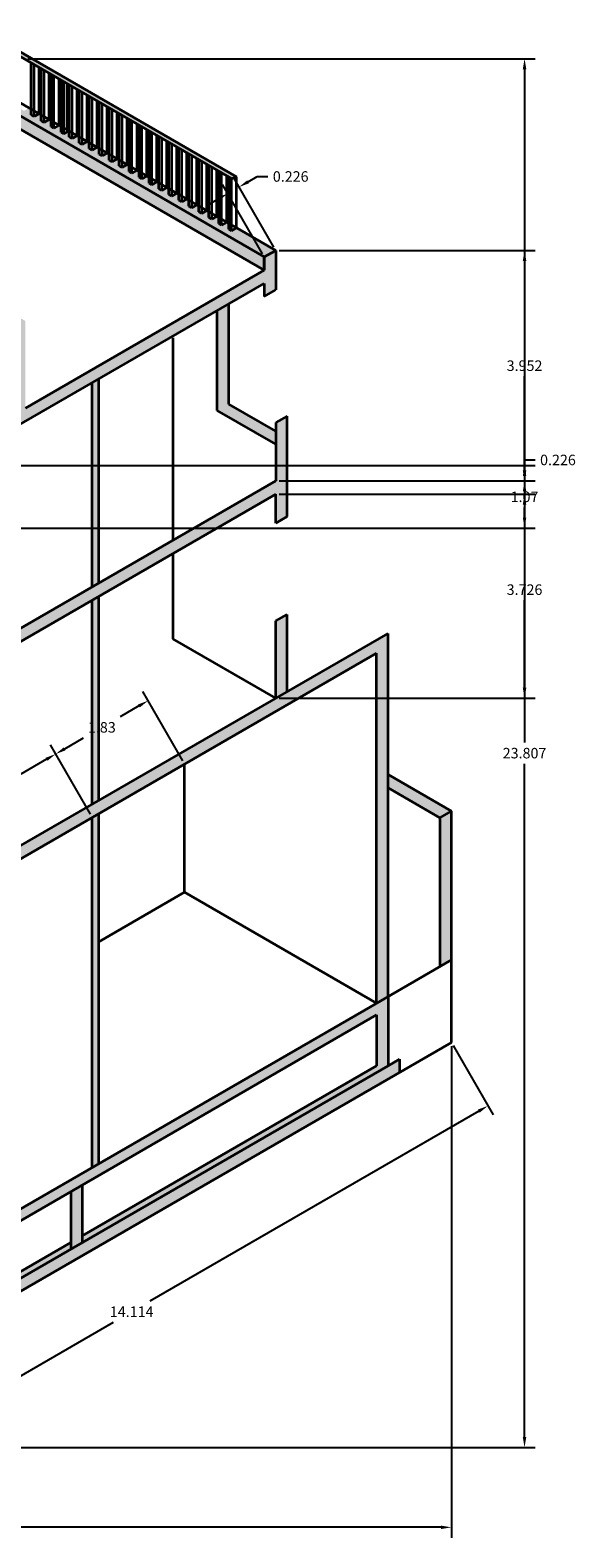
# Model space of a CAD drawing. Units: metres. Extents: x 26125 to 52281, y 14233 to 28508.
# Tile 4 of 4: x 26142 to 26151, y 14233 to 14259. Entities that reach past the tile are written whole.
import ezdxf

# ---------------------------------------------------------------- set-up
doc = ezdxf.new("R2010")
doc.units = ezdxf.units.M
for name, color, linetype, lineweight in [('A-ANNO-DIMS', 2, 'Continuous', 18), ('A-ELEV-PATT', 32, 'Continuous', 13), ('A-WALL', 7, 'Continuous', 35), ('A-WALL-PATT', 9, 'Continuous', 13)]:
    doc.layers.add(name, color=color, linetype=linetype, lineweight=lineweight)
doc.styles.get("Standard").update_dxf_attribs({"font": 'arial.ttf'})
doc.dimstyles.get("Standard").update_dxf_attribs({"dimtxt": 0.18, "dimasz": 0.18, "dimexe": 0.18, "dimexo": 0.0625, "dimgap": 0.09, "dimtad": 0, "dimtih": 1, "dimtoh": 1, "dimdec": 4, "dimzin": 0, "dimdsep": 46, "dimtxsty": 'Standard', "dimcen": 0.09, "dimadec": 0, "dimazin": 0, "dimtfac": 1, "dimtdec": 4, "dimtofl": 0, "dimtmove": 0, "dimatfit": 3, "dimfxl": 1, "dimtolj": 1, "dimtzin": 0, "dimarcsym": 0})

# ---------------------------------------------------------------- blocks, each defined once
blk = doc.blocks.new('*D10')
at = {"layer": 'A-ANNO-DIMS', "color": 0, "lineweight": -2, "transparency": 16777216}
for p, q in [((26148.791, 14241.887), (26148.791, 14233.458)), ((26126.609, 14240.579), (26126.609, 14233.458)), ((26126.789, 14233.638), (26137.305, 14233.638)), ((26148.611, 14233.638), (26138.096, 14233.638))]:
    blk.add_line(p, q, dxfattribs=at)
at = {"layer": 'A-ANNO-DIMS', "color": 0, "transparency": 16777216}
for points in [[(26126.789, 14233.668), (26126.789, 14233.608), (26126.609, 14233.638)], [(26148.611, 14233.668), (26148.611, 14233.608), (26148.791, 14233.638)]]:
    blk.add_solid(points, dxfattribs=at)
at = {"layer": 'Defpoints', "color": 0, "transparency": 16777216}
for p in [(26148.791, 14241.95), (26126.609, 14240.642), (26148.791, 14233.638)]:
    blk.add_point(p, dxfattribs=at)
at = {"layer": 'A-ANNO-DIMS', "color": 0, "transparency": 16777216, "insert": (26137.7, 14233.638), "char_height": 0.18, "attachment_point": 5}
blk.add_mtext('\\A1;22.18', dxfattribs=at)
blk = doc.blocks.new('*D11')
at = {"layer": 'A-ANNO-DIMS', "color": 0, "lineweight": -2, "transparency": 16777216}
for p, q in [((26141.524, 14258.813), (26150.226, 14258.813)), ((26150.046, 14258.633), (26150.046, 14247.091)), ((26150.046, 14235.186), (26150.046, 14246.727)), ((26136.826, 14235.006), (26150.226, 14235.006))]:
    blk.add_line(p, q, dxfattribs=at)
at = {"layer": 'A-ANNO-DIMS', "color": 0, "transparency": 16777216}
for points in [[(26150.016, 14258.633), (26150.076, 14258.633), (26150.046, 14258.813)], [(26150.016, 14235.186), (26150.076, 14235.186), (26150.046, 14235.006)]]:
    blk.add_solid(points, dxfattribs=at)
at = {"layer": 'Defpoints', "color": 0, "transparency": 16777216}
for p in [(26141.462, 14258.813), (26150.046, 14258.813), (26136.763, 14235.006)]:
    blk.add_point(p, dxfattribs=at)
at = {"layer": 'A-ANNO-DIMS', "color": 0, "transparency": 16777216, "insert": (26150.046, 14246.909), "char_height": 0.18, "attachment_point": 5}
blk.add_mtext('\\A1;23.807', dxfattribs=at)
blk = doc.blocks.new('*D13')
at = {"layer": 'A-ANNO-DIMS', "color": 0, "lineweight": -2, "transparency": 16777216}
for p, q in [((26148.822, 14241.896), (26149.508, 14240.707)), ((26149.262, 14240.773), (26143.619, 14237.515)), ((26137.351, 14233.896), (26142.994, 14237.154)), ((26136.599, 14234.838), (26137.285, 14233.65))]:
    blk.add_line(p, q, dxfattribs=at)
at = {"layer": 'A-ANNO-DIMS', "color": 0, "transparency": 16777216}
for points in [[(26149.247, 14240.799), (26149.277, 14240.747), (26149.418, 14240.863)], [(26137.336, 14233.922), (26137.366, 14233.87), (26137.195, 14233.806)]]:
    blk.add_solid(points, dxfattribs=at)
at = {"layer": 'Defpoints', "color": 0, "transparency": 16777216}
for p in [(26148.791, 14241.95), (26136.568, 14234.893), (26137.195, 14233.806)]:
    blk.add_point(p, dxfattribs=at)
at = {"layer": 'A-ANNO-DIMS', "color": 0, "transparency": 16777216, "insert": (26143.307, 14237.334), "char_height": 0.18, "attachment_point": 5}
blk.add_mtext('\\A1;14.114', dxfattribs=at)
blk = doc.blocks.new('*D15')
at = {"layer": 'A-ANNO-DIMS', "color": 0, "lineweight": -2, "transparency": 16777216}
for p, q in [((26150.046, 14251.755), (26150.046, 14251.935)), ((26150.046, 14251.935), (26150.226, 14251.935)), ((26145.84, 14251.575), (26150.226, 14251.575)), ((26145.84, 14251.349), (26150.226, 14251.349)), ((26150.046, 14251.169), (26150.046, 14250.989))]:
    blk.add_line(p, q, dxfattribs=at)
at = {"layer": 'A-ANNO-DIMS', "color": 0, "transparency": 16777216}
for points in [[(26150.016, 14251.755), (26150.076, 14251.755), (26150.046, 14251.575)], [(26150.016, 14251.169), (26150.076, 14251.169), (26150.046, 14251.349)]]:
    blk.add_solid(points, dxfattribs=at)
at = {"layer": 'Defpoints', "color": 0, "transparency": 16777216}
for p in [(26145.777, 14251.575), (26150.046, 14251.575), (26145.777, 14251.349)]:
    blk.add_point(p, dxfattribs=at)
at = {"layer": 'A-ANNO-DIMS', "color": 0, "transparency": 16777216, "insert": (26150.619, 14251.935), "char_height": 0.18, "attachment_point": 5}
blk.add_mtext('\\A1;0.226', dxfattribs=at)
blk = doc.blocks.new('*D16')
at = {"layer": 'A-ANNO-DIMS', "color": 0, "lineweight": -2, "transparency": 16777216}
for p, q in [((26145.55, 14255.468), (26144.864, 14256.657)), ((26145.746, 14255.581), (26145.06, 14256.77)), ((26145.306, 14256.704), (26145.462, 14256.794)), ((26145.462, 14256.794), (26145.642, 14256.794)), ((26144.798, 14256.411), (26144.642, 14256.321))]:
    blk.add_line(p, q, dxfattribs=at)
at = {"layer": 'A-ANNO-DIMS', "color": 0, "transparency": 16777216}
for points in [[(26145.291, 14256.73), (26145.321, 14256.678), (26145.15, 14256.614)], [(26144.783, 14256.437), (26144.813, 14256.385), (26144.954, 14256.501)]]:
    blk.add_solid(points, dxfattribs=at)
at = {"layer": 'Defpoints', "color": 0, "transparency": 16777216}
for p in [(26145.15, 14256.614), (26145.582, 14255.414), (26145.777, 14255.527)]:
    blk.add_point(p, dxfattribs=at)
at = {"layer": 'A-ANNO-DIMS', "color": 0, "transparency": 16777216, "insert": (26146.035, 14256.794), "char_height": 0.18, "attachment_point": 5}
blk.add_mtext('\\A1;0.226', dxfattribs=at)
blk = doc.blocks.new('*D17')
at = {"layer": 'A-ANNO-DIMS', "color": 0, "lineweight": -2, "transparency": 16777216}
for p, q in [((26145.84, 14251.575), (26150.226, 14251.575)), ((26150.046, 14251.395), (26150.046, 14249.894)), ((26150.046, 14248.029), (26150.046, 14249.53)), ((26145.84, 14247.849), (26150.226, 14247.849))]:
    blk.add_line(p, q, dxfattribs=at)
at = {"layer": 'A-ANNO-DIMS', "color": 0, "transparency": 16777216}
for points in [[(26150.016, 14251.395), (26150.076, 14251.395), (26150.046, 14251.575)], [(26150.016, 14248.029), (26150.076, 14248.029), (26150.046, 14247.849)]]:
    blk.add_solid(points, dxfattribs=at)
at = {"layer": 'Defpoints', "color": 0, "transparency": 16777216}
for p in [(26145.777, 14251.575), (26150.046, 14251.575), (26145.777, 14247.849)]:
    blk.add_point(p, dxfattribs=at)
at = {"layer": 'A-ANNO-DIMS', "color": 0, "transparency": 16777216, "insert": (26150.046, 14249.712), "char_height": 0.18, "attachment_point": 5}
blk.add_mtext('\\A1;3.726', dxfattribs=at)
blk = doc.blocks.new('*D18')
at = {"layer": 'A-ANNO-DIMS', "color": 0, "lineweight": -2, "transparency": 16777216}
for p, q in [((26145.84, 14255.527), (26150.226, 14255.527)), ((26150.046, 14255.347), (26150.046, 14253.733)), ((26150.046, 14251.755), (26150.046, 14253.369)), ((26145.84, 14251.575), (26150.226, 14251.575))]:
    blk.add_line(p, q, dxfattribs=at)
at = {"layer": 'A-ANNO-DIMS', "color": 0, "transparency": 16777216}
for points in [[(26150.016, 14255.347), (26150.076, 14255.347), (26150.046, 14255.527)], [(26150.016, 14251.755), (26150.076, 14251.755), (26150.046, 14251.575)]]:
    blk.add_solid(points, dxfattribs=at)
at = {"layer": 'Defpoints', "color": 0, "transparency": 16777216}
for p in [(26145.777, 14255.527), (26150.046, 14255.527), (26145.777, 14251.575)]:
    blk.add_point(p, dxfattribs=at)
at = {"layer": 'A-ANNO-DIMS', "color": 0, "transparency": 16777216, "insert": (26150.046, 14253.551), "char_height": 0.18, "attachment_point": 5}
blk.add_mtext('\\A1;3.952', dxfattribs=at)
blk = doc.blocks.new('*D22')
at = {"layer": 'A-ANNO-DIMS', "color": 0, "lineweight": -2, "transparency": 16777216}
for p, q in [((26137.988, 14251.837), (26150.226, 14251.837)), ((26150.046, 14251.657), (26150.046, 14251.485)), ((26150.046, 14250.948), (26150.046, 14251.121)), ((26137.988, 14250.768), (26150.226, 14250.768))]:
    blk.add_line(p, q, dxfattribs=at)
at = {"layer": 'A-ANNO-DIMS', "color": 0, "transparency": 16777216}
for points in [[(26150.016, 14251.657), (26150.076, 14251.657), (26150.046, 14251.837)], [(26150.016, 14250.948), (26150.076, 14250.948), (26150.046, 14250.768)]]:
    blk.add_solid(points, dxfattribs=at)
at = {"layer": 'Defpoints', "color": 0, "transparency": 16777216}
for p in [(26137.925, 14251.837), (26137.925, 14250.768), (26150.046, 14250.768)]:
    blk.add_point(p, dxfattribs=at)
at = {"layer": 'A-ANNO-DIMS', "color": 0, "transparency": 16777216, "insert": (26150.046, 14251.303), "char_height": 0.18, "attachment_point": 5}
blk.add_mtext('\\A1;1.07', dxfattribs=at)
blk = doc.blocks.new('*D30')
at = {"layer": 'A-ANNO-DIMS', "color": 0, "lineweight": -2, "transparency": 16777216}
for p, q in [((26142.6, 14245.861), (26141.913, 14247.049)), ((26141.847, 14246.803), (26141.404, 14246.547)), ((26140.77, 14244.804), (26140.083, 14245.993)), ((26140.329, 14245.927), (26140.773, 14246.183))]:
    blk.add_line(p, q, dxfattribs=at)
at = {"layer": 'A-ANNO-DIMS', "color": 0, "transparency": 16777216}
for points in [[(26141.832, 14246.829), (26141.862, 14246.777), (26142.003, 14246.893)], [(26140.314, 14245.953), (26140.344, 14245.901), (26140.173, 14245.837)]]:
    blk.add_solid(points, dxfattribs=at)
at = {"layer": 'Defpoints', "color": 0, "transparency": 16777216}
for p in [(26142.003, 14246.893), (26142.631, 14245.807), (26140.801, 14244.75)]:
    blk.add_point(p, dxfattribs=at)
at = {"layer": 'A-ANNO-DIMS', "color": 0, "transparency": 16777216, "insert": (26141.088, 14246.365), "char_height": 0.18, "attachment_point": 5}
blk.add_mtext('\\A1;2.113', dxfattribs=at)
blk = doc.blocks.new('*D31')
at = {"layer": 'A-ANNO-DIMS', "color": 0, "lineweight": -2, "transparency": 16777216}
for p, q in [((26144.184, 14246.776), (26143.498, 14247.964)), ((26143.432, 14247.718), (26143.111, 14247.533)), ((26142.6, 14245.861), (26141.913, 14247.049)), ((26142.159, 14246.983), (26142.481, 14247.169))]:
    blk.add_line(p, q, dxfattribs=at)
at = {"layer": 'A-ANNO-DIMS', "color": 0, "transparency": 16777216}
for points in [[(26143.417, 14247.744), (26143.447, 14247.692), (26143.588, 14247.808)], [(26142.144, 14247.009), (26142.174, 14246.957), (26142.003, 14246.893)]]:
    blk.add_solid(points, dxfattribs=at)
at = {"layer": 'Defpoints', "color": 0, "transparency": 16777216}
for p in [(26143.588, 14247.808), (26144.216, 14246.722), (26142.631, 14245.807)]:
    blk.add_point(p, dxfattribs=at)
at = {"layer": 'A-ANNO-DIMS', "color": 0, "transparency": 16777216, "insert": (26142.796, 14247.351), "char_height": 0.18, "attachment_point": 5}
blk.add_mtext('\\A1;1.83', dxfattribs=at)

msp = doc.modelspace()

# ---------------------------------------------------------------- hatches: boundary and pattern name
at = {"layer": 'A-ELEV-PATT'}
h = msp.add_hatch(color=256, dxfattribs=at)
h.dxf.hatch_style = 1
h.paths.add_polyline_path([(26139.7617, 14247.876), (26139.6635, 14247.8193), (26139.6635, 14244.3193), (26139.7617, 14244.376)])
h.paths.add_polyline_path([(26134.1363, 14247.6744), (26134.0497, 14247.7244), (26134.0497, 14244.7066), (26134.1363, 14244.7566)])
h.paths.add_polyline_path([(26135.2033, 14244.0405), (26135.3053, 14244.1136), (26135.3053, 14246.9994), (26135.2033, 14247.0583)])
h.paths.add_polyline_path([(26140.8009, 14238.75), (26140.8988, 14238.8065), (26140.8988, 14244.8065), (26140.8009, 14244.75)])
h.paths.add_polyline_path([(26142.7463, 14245.8732), (26142.6308, 14245.8065), (26142.6308, 14239.8065), (26142.7463, 14239.8732)])
h.paths.add_polyline_path([(26142.7463, 14249.5992), (26142.6308, 14249.5325), (26142.6308, 14246.0325), (26142.7463, 14246.0992)])
h.paths.add_polyline_path([(26140.8009, 14244.976), (26140.8988, 14245.0325), (26140.8988, 14248.5325), (26140.8009, 14248.476)])
h.paths.add_polyline_path([(26142.6308, 14249.7585), (26142.7463, 14249.8252), (26142.7463, 14253.3252), (26142.6308, 14253.2585)])
h.paths.add_polyline_path([(26136.4442, 14251.397), (26136.3576, 14251.447), (26136.3576, 14248.5341), (26136.4442, 14248.4841)])
at = {"layer": 'A-WALL-PATT'}
h = msp.add_hatch(color=256, dxfattribs=at)
h.dxf.hatch_style = 1
h.paths.add_polyline_path([(26132.7127, 14248.4963), (26132.7127, 14248.7223), (26131.6604, 14248.1148), (26131.6604, 14247.8888)])
h.paths.add_polyline_path([(26132.7127, 14248.7223), (26132.7127, 14248.4963), (26136.7743, 14246.1513), (26136.7743, 14246.3773)])
h.paths.add_polyline_path([(26145.7774, 14251.3492), (26145.7774, 14250.8522), (26145.9732, 14250.9652), (26145.9732, 14251.6882), (26145.9732, 14252.3156), (26145.7774, 14252.4288), (26145.7774, 14251.5752), (26136.7743, 14246.3773), (26136.7743, 14246.1513), (26136.97, 14246.2643), (26136.97, 14246.1509), (26137.1658, 14246.2639), (26137.1658, 14246.3773)])
h.paths.add_polyline_path([(26135.3545, 14249.1132), (26135.1588, 14249.0002), (26138.2381, 14247.2224), (26138.4338, 14247.3354)])
h.paths.add_polyline_path([(26135.3545, 14252.0261), (26135.1588, 14252.1391), (26135.1588, 14249.0002), (26135.3545, 14249.1132)])
h.paths.add_polyline_path([(26137.9254, 14251.8375), (26137.7296, 14251.7245), (26137.7296, 14250.6548), (26137.9254, 14250.7678)], flags=17)
h.paths.add_polyline_path([(26144.9726, 14252.8939), (26144.9726, 14254.6106), (26144.7764, 14254.4973), (26144.7764, 14252.7806), (26145.7774, 14252.2026), (26145.7774, 14252.4288)])
h.paths.add_polyline_path([(26147.5095, 14248.6232), (26147.5095, 14242.6232), (26147.7052, 14242.7362), (26147.7052, 14248.9622), (26136.1883, 14242.3129), (26136.1883, 14242.0869), (26136.97, 14242.5383), (26136.97, 14242.3123), (26137.1658, 14242.4253), (26137.1658, 14242.6513)])
h.paths.add_polyline_path([(26145.9732, 14249.2872), (26145.7774, 14249.1742), (26145.7774, 14247.8492), (26145.9732, 14247.9622)], flags=17)
h.paths.add_polyline_path([(26145.5817, 14254.9622), (26145.5817, 14254.7362), (26145.7774, 14254.8492), (26145.7774, 14255.5272), (26145.5817, 14255.4142), (26145.5817, 14255.1882), (26141.4857, 14252.8234), (26141.4857, 14252.5974)])
h.paths.add_polyline_path([(26140.5667, 14258.3096), (26140.5667, 14258.0836), (26145.5817, 14255.1882), (26145.5817, 14255.4142)])
h.paths.add_polyline_path([(26140.7524, 14259.0772), (26140.7524, 14259.3025), (26137.3207, 14257.3212), (26137.5157, 14257.2086)])
h.paths.add_polyline_path([(26138.0751, 14255.9856), (26138.3349, 14256.1356), (26138.5947, 14255.9856), (26138.5947, 14256.5856), (26138.0751, 14256.2856), (26134.148, 14254.0183), (26134.4078, 14253.8683)])
h.paths.add_polyline_path([(26140.5667, 14258.0836), (26140.5667, 14258.3096), (26140.7524, 14258.4285), (26140.7524, 14259.0772), (26137.5157, 14257.2086), (26138.2834, 14256.7653)])
h.paths.add_polyline_path([(26145.1083, 14255.9136), (26145.0216, 14255.8636), (26144.9721, 14255.8922), (26144.9721, 14255.9922), (26144.9373, 14256.0123), (26144.8507, 14255.9623), (26144.8012, 14255.9909), (26144.8012, 14256.0909), (26144.7664, 14256.1109), (26144.6798, 14256.0609), (26144.6303, 14256.0896), (26144.6303, 14256.1896), (26144.5955, 14256.2096), (26144.5089, 14256.1596), (26144.4594, 14256.1882), (26144.4594, 14256.2882), (26144.4246, 14256.3083), (26144.338, 14256.2583), (26144.2885, 14256.2869), (26144.2885, 14256.3869), (26144.2537, 14256.407), (26144.1671, 14256.357), (26144.1176, 14256.3856), (26144.1176, 14256.4856), (26144.0828, 14256.5056), (26143.9962, 14256.4556), (26143.9466, 14256.4842), (26143.9466, 14256.5842), (26143.9119, 14256.6043), (26143.8253, 14256.5543), (26143.7757, 14256.5829), (26143.7757, 14256.6829), (26143.741, 14256.703), (26143.6544, 14256.653), (26143.6048, 14256.6816), (26143.6048, 14256.7816), (26143.5701, 14256.8017), (26143.4835, 14256.7517), (26143.4339, 14256.7803), (26143.4339, 14256.8803), (26143.3992, 14256.9003), (26143.3126, 14256.8503), (26143.263, 14256.8789), (26143.263, 14256.9789), (26143.2283, 14256.999), (26143.1417, 14256.949), (26143.0921, 14256.9776), (26143.0921, 14257.0776), (26143.0573, 14257.0977), (26142.9707, 14257.0477), (26142.9212, 14257.0763), (26142.9212, 14257.1763), (26142.8864, 14257.1964), (26142.7998, 14257.1464), (26142.7503, 14257.175), (26142.7503, 14257.275), (26142.7155, 14257.295), (26142.6289, 14257.245), (26142.5794, 14257.2736), (26142.5794, 14257.3736), (26142.5446, 14257.3937), (26142.458, 14257.3437), (26142.4085, 14257.3723), (26142.4085, 14257.4723), (26142.3737, 14257.4924), (26142.2871, 14257.4424), (26142.2376, 14257.471), (26142.2376, 14257.571), (26142.2322, 14257.5741), (26142.1456, 14257.5241), (26142.0961, 14257.5527), (26142.0961, 14257.6527), (26142.0613, 14257.6727), (26141.9747, 14257.6227), (26141.9252, 14257.6514), (26141.9252, 14257.7514), (26141.8904, 14257.7714), (26141.8038, 14257.7214), (26141.7542, 14257.75), (26141.7542, 14257.85), (26141.7195, 14257.8701), (26141.6329, 14257.8201), (26141.5833, 14257.8487), (26141.5833, 14257.9487), (26141.5486, 14257.9688), (26141.462, 14257.9188), (26141.4124, 14257.9474), (26141.4124, 14258.0474), (26141.3777, 14258.0674), (26141.2911, 14258.0174), (26141.2415, 14258.0461), (26141.2415, 14258.1461), (26141.2068, 14258.1661), (26141.1202, 14258.1161), (26141.0706, 14258.1447), (26141.0706, 14258.2447), (26141.0359, 14258.2648), (26140.9493, 14258.2148), (26140.8997, 14258.2434), (26140.8997, 14258.3434), (26140.8885, 14258.3499), (26140.8019, 14258.2999), (26140.7524, 14258.3285), (26140.7524, 14258.4285), (26140.5667, 14258.3096), (26145.5817, 14255.4142), (26145.7774, 14255.5272)])
h.paths.add_polyline_path([(26141.4857, 14254.3165), (26141.3093, 14254.2146), (26141.3093, 14252.4955), (26141.4857, 14252.5974)])
h.paths.add_polyline_path([(26140.2525, 14255.0285), (26140.0568, 14254.9155), (26141.29, 14254.2035), (26141.4857, 14254.3165)])
h = msp.add_hatch(color=256, dxfattribs=at)
h.dxf.hatch_style = 1
h.paths.add_polyline_path([(26140.7524, 14259.3025), (26140.7524, 14259.2223), (26145.0216, 14256.7575), (26145.1083, 14256.7876)])
h = msp.add_hatch(color=256, dxfattribs=at)
h.dxf.hatch_style = 1
h.paths.add_polyline_path([(26145.9732, 14252.6882), (26145.7774, 14252.5752), (26145.7774, 14252.4288), (26145.9732, 14252.3156)])
h = msp.add_hatch(color=256, dxfattribs=at)
h.dxf.hatch_style = 1
h.paths.add_polyline_path([(26148.7909, 14245.9139), (26148.5951, 14245.8009), (26148.5951, 14243.25), (26148.7909, 14243.363)])
h.paths.add_polyline_path([(26147.7052, 14246.5407), (26147.7052, 14246.3147), (26148.5951, 14245.8009), (26148.7909, 14245.9139)])
h = msp.add_hatch(color=256, dxfattribs=at)
h.dxf.hatch_style = 1
h.paths.add_polyline_path([(26126.9422, 14241.8758), (26126.7465, 14241.7628), (26136.5676, 14236.0925), (26136.7633, 14236.2055)])
h.paths.add_polyline_path([(26126.7465, 14241.7628), (26126.7318, 14241.7712), (26126.7318, 14244.7755), (26126.6095, 14244.8461), (26126.6095, 14240.6418), (26136.5676, 14234.8925), (26136.5676, 14236.0925)])
h.paths.add_polyline_path([(26138.4953, 14236.3449), (26138.4953, 14237.2055), (26136.7633, 14236.2055), (26136.7633, 14235.0055), (26138.2239, 14235.8488), (26138.1257, 14235.9055), (26138.1257, 14236.1315)])
h.paths.add_polyline_path([(26140.7034, 14237.2803), (26147.9009, 14241.4358), (26147.9009, 14241.6618), (26147.7052, 14241.5488), (26140.6052, 14237.4496), (26138.2239, 14236.0748), (26138.2239, 14235.8488)])
h.paths.add_polyline_path([(26140.6052, 14237.4496), (26142.2637, 14238.4072), (26142.2637, 14238.5206), (26138.6911, 14236.4579), (26138.6911, 14236.3445)], flags=17)
h.paths.add_polyline_path([(26138.4953, 14236.2315), (26138.4953, 14236.3449), (26138.1257, 14236.1315), (26138.2239, 14236.0748)], flags=17)
h.paths.add_polyline_path([(26138.2239, 14236.0748), (26138.1257, 14236.1315), (26138.1257, 14235.9055), (26138.2239, 14235.8488)], flags=17)
h.paths.add_polyline_path([(26136.7633, 14236.2055), (26136.5676, 14236.0925), (26136.5676, 14234.8925), (26136.7633, 14235.0055)])
h.paths.add_polyline_path([(26138.4953, 14237.2055), (26138.2996, 14237.3185), (26136.5676, 14236.3185), (26136.7633, 14236.2055)])
h.paths.add_polyline_path([(26128.558, 14246.2845), (26128.2718, 14246.1192), (26131.4647, 14244.2758), (26131.4647, 14244.6063)])
h.paths.add_polyline_path([(26128.2234, 14245.6367), (26128.2234, 14245.7792), (26126.6095, 14244.8474), (26126.6095, 14244.8461), (26126.7318, 14244.7755)])
h = msp.add_hatch(color=256, dxfattribs=at)
h.dxf.hatch_style = 1
h.paths.add_polyline_path([(26147.7052, 14242.7362), (26147.2961, 14242.5), (26142.7463, 14239.8732), (26142.7463, 14239.6732), (26147.5095, 14242.4232), (26147.5095, 14241.5492), (26142.4594, 14238.6336), (26142.4594, 14238.5202), (26147.7052, 14241.5488)])
h = msp.add_hatch(color=256, dxfattribs=at)
h.dxf.hatch_style = 1
h.paths.add_polyline_path([(26147.5095, 14242.4232), (26147.5095, 14241.5492), (26142.4594, 14238.6336), (26142.4594, 14238.5202), (26147.7052, 14241.5488), (26147.7052, 14242.5102), (26147.5095, 14242.6232), (26147.2961, 14242.5), (26142.7463, 14239.8732), (26142.7463, 14239.6732)])
h.paths.add_polyline_path([(26142.7463, 14239.6732), (26142.7463, 14239.8732), (26138.4953, 14237.4189), (26138.4953, 14237.2189)])
h.paths.add_polyline_path([(26142.4594, 14239.5076), (26142.2637, 14239.3946), (26142.2637, 14238.4072), (26142.4594, 14238.5202), (26142.4594, 14238.6336)], flags=17)
h.paths.add_polyline_path([(26138.6911, 14237.3319), (26138.4953, 14237.2189), (26138.4953, 14236.2315), (26138.6911, 14236.3445)])

# ---------------------------------------------------------------- linework, layer by layer
at = {"layer": 'A-WALL'}
for p, q in [((26140.7524, 14259.3025), (26145.1083, 14256.7876)), ((26140.7524, 14259.2223), (26145.0216, 14256.7575)), ((26141.5833, 14257.8487), (26141.5833, 14258.7426)), ((26141.6329, 14257.8201), (26141.6329, 14258.714)), ((26141.7195, 14257.8701), (26141.7195, 14258.664)), ((26145.7774, 14255.5272), (26140.7524, 14258.4285)), ((26141.7542, 14257.75), (26141.7542, 14258.6439)), ((26141.8038, 14257.7214), (26141.8038, 14258.6153)), ((26141.8904, 14257.7714), (26141.8904, 14258.5653)), ((26141.9252, 14257.6514), (26141.9252, 14258.5452)), ((26141.9747, 14257.6227), (26141.9747, 14258.5166)), ((26142.0613, 14257.6727), (26142.0613, 14258.4666)), ((26142.0961, 14257.5527), (26142.0961, 14258.4466)), ((26142.1456, 14257.5241), (26142.1456, 14258.4179)), ((26140.5667, 14258.3096), (26145.5817, 14255.4142)), ((26142.2028, 14257.5911), (26142.2028, 14258.3849)), ((26142.2376, 14257.471), (26142.2376, 14258.3649)), ((26142.2871, 14257.4424), (26142.2871, 14258.3363)), ((26142.3737, 14257.4924), (26142.3737, 14258.2863)), ((26142.4085, 14257.3723), (26142.4085, 14258.2662)), ((26142.458, 14257.3437), (26142.458, 14258.2376)), ((26142.5446, 14257.3937), (26142.5446, 14258.1876)), ((26142.5794, 14257.2736), (26142.5794, 14258.1675)), ((26142.6289, 14257.245), (26142.6289, 14258.1389)), ((26145.5817, 14255.1882), (26140.5667, 14258.0836)), ((26142.7155, 14257.295), (26142.7155, 14258.0889)), ((26142.7503, 14257.175), (26142.7503, 14258.0688)), ((26142.7998, 14257.1464), (26142.7998, 14258.0402)), ((26142.8864, 14257.1964), (26142.8864, 14257.9902)), ((26142.9212, 14257.0763), (26142.9212, 14257.9702)), ((26142.9707, 14257.0477), (26142.9707, 14257.9416)), ((26143.0573, 14257.0977), (26143.0573, 14257.8916)), ((26141.6329, 14257.8201), (26141.5833, 14257.8487)), ((26141.7195, 14257.8701), (26141.6329, 14257.8201)), ((26141.8038, 14257.7214), (26141.7542, 14257.75)), ((26141.8904, 14257.7714), (26141.8038, 14257.7214)), ((26141.9747, 14257.6227), (26141.9252, 14257.6514)), ((26142.0613, 14257.6727), (26141.9747, 14257.6227)), ((26143.0921, 14256.9776), (26143.0921, 14257.8715)), ((26143.1417, 14256.949), (26143.1417, 14257.8429)), ((26143.2283, 14256.999), (26143.2283, 14257.7929)), ((26143.263, 14256.8789), (26143.263, 14257.7728)), ((26143.3126, 14256.8503), (26143.3126, 14257.7442)), ((26143.3992, 14256.9003), (26143.3992, 14257.6942)), ((26143.4339, 14256.7803), (26143.4339, 14257.6741)), ((26143.4835, 14256.7517), (26143.4835, 14257.6455)), ((26142.1456, 14257.5241), (26142.0961, 14257.5527)), ((26142.2322, 14257.5741), (26142.1456, 14257.5241)), ((26142.2871, 14257.4424), (26142.2376, 14257.471)), ((26142.3737, 14257.4924), (26142.2871, 14257.4424)), ((26142.458, 14257.3437), (26142.4085, 14257.3723)), ((26142.5446, 14257.3937), (26142.458, 14257.3437)), ((26143.5701, 14256.8017), (26143.5701, 14257.5955)), ((26143.6048, 14256.6816), (26143.6048, 14257.5755)), ((26143.6544, 14256.653), (26143.6544, 14257.5469)), ((26143.741, 14256.703), (26143.741, 14257.4969)), ((26143.7757, 14256.5829), (26143.7757, 14257.4768)), ((26143.8253, 14256.5543), (26143.8253, 14257.4482)), ((26143.9119, 14256.6043), (26143.9119, 14257.3982)), ((26143.9466, 14256.4842), (26143.9466, 14257.3781)), ((26142.6289, 14257.245), (26142.5794, 14257.2736)), ((26142.7155, 14257.295), (26142.6289, 14257.245)), ((26142.7998, 14257.1464), (26142.7503, 14257.175)), ((26142.8864, 14257.1964), (26142.7998, 14257.1464)), ((26143.9962, 14256.4556), (26143.9962, 14257.3495)), ((26144.0828, 14256.5056), (26144.0828, 14257.2995)), ((26144.1176, 14256.3856), (26144.1176, 14257.2794)), ((26144.1671, 14256.357), (26144.1671, 14257.2508)), ((26144.2537, 14256.407), (26144.2537, 14257.2008)), ((26144.2885, 14256.2869), (26144.2885, 14257.1808)), ((26144.338, 14256.2583), (26144.338, 14257.1522)), ((26144.4246, 14256.3083), (26144.4246, 14257.1022)), ((26142.9707, 14257.0477), (26142.9212, 14257.0763)), ((26143.0573, 14257.0977), (26142.9707, 14257.0477)), ((26143.1417, 14256.949), (26143.0921, 14256.9776)), ((26143.2283, 14256.999), (26143.1417, 14256.949)), ((26143.3126, 14256.8503), (26143.263, 14256.8789)), ((26143.3992, 14256.9003), (26143.3126, 14256.8503)), ((26144.4594, 14256.1882), (26144.4594, 14257.0821)), ((26144.5089, 14256.1596), (26144.5089, 14257.0535)), ((26144.5955, 14256.2096), (26144.5955, 14257.0035)), ((26144.6303, 14256.0896), (26144.6303, 14256.9834)), ((26144.6798, 14256.0609), (26144.6798, 14256.9548)), ((26144.7664, 14256.1109), (26144.7664, 14256.9048)), ((26144.8012, 14255.9909), (26144.8012, 14256.8848)), ((26144.8507, 14255.9623), (26144.8507, 14256.8561)), ((26143.4835, 14256.7517), (26143.4339, 14256.7803)), ((26143.5701, 14256.8017), (26143.4835, 14256.7517)), ((26143.6544, 14256.653), (26143.6048, 14256.6816)), ((26143.741, 14256.703), (26143.6544, 14256.653)), ((26143.8253, 14256.5543), (26143.7757, 14256.5829)), ((26143.9119, 14256.6043), (26143.8253, 14256.5543)), ((26144.9373, 14256.0123), (26144.9373, 14256.8061)), ((26144.9721, 14255.8922), (26144.9721, 14256.7861)), ((26145.0216, 14256.7575), (26145.1083, 14256.7876)), ((26145.0216, 14255.8636), (26145.0216, 14256.7575)), ((26145.1083, 14255.9136), (26145.1083, 14256.7876)), ((26143.9962, 14256.4556), (26143.9466, 14256.4842)), ((26144.0828, 14256.5056), (26143.9962, 14256.4556)), ((26144.1671, 14256.357), (26144.1176, 14256.3856)), ((26144.2537, 14256.407), (26144.1671, 14256.357)), ((26144.338, 14256.2583), (26144.2885, 14256.2869)), ((26144.4246, 14256.3083), (26144.338, 14256.2583)), ((26144.5089, 14256.1596), (26144.4594, 14256.1882)), ((26144.5955, 14256.2096), (26144.5089, 14256.1596)), ((26144.6798, 14256.0609), (26144.6303, 14256.0896)), ((26144.7664, 14256.1109), (26144.6798, 14256.0609)), ((26144.8507, 14255.9623), (26144.8012, 14255.9909)), ((26144.9373, 14256.0123), (26144.8507, 14255.9623)), ((26145.0216, 14255.8636), (26144.9721, 14255.8922)), ((26145.1083, 14255.9136), (26145.0216, 14255.8636)), ((26145.5817, 14255.4142), (26145.7774, 14255.5272)), ((26145.5817, 14255.1882), (26145.5817, 14255.4142)), ((26145.5817, 14255.4142), (26145.5817, 14255.1882)), ((26145.7774, 14255.5272), (26145.7774, 14254.8492)), ((26141.4857, 14252.8234), (26145.5817, 14255.1882)), ((26141.3093, 14252.4955), (26145.5817, 14254.9622)), ((26145.5817, 14254.9622), (26145.5817, 14254.7362)), ((26145.5817, 14254.7362), (26145.7774, 14254.8492)), ((26144.9726, 14252.8939), (26144.9726, 14254.6106)), ((26144.7764, 14252.7806), (26144.7764, 14254.4973)), ((26144.0122, 14254.0292), (26144.0122, 14250.5561)), ((26142.6308, 14249.7585), (26142.6308, 14253.2585)), ((26142.7463, 14249.8252), (26142.7463, 14253.3252)), ((26145.7774, 14252.2026), (26144.7764, 14252.7806)), ((26145.7774, 14252.4288), (26144.9726, 14252.8939)), ((26145.9732, 14252.6882), (26145.7774, 14252.5752)), ((26145.7774, 14252.5752), (26145.7774, 14251.5752)), ((26145.9732, 14251.6882), (26145.9732, 14252.6882)), ((26145.9737, 14252.5892), (26145.9732, 14252.5895)), ((26145.9732, 14250.9652), (26145.9732, 14251.6882)), ((26136.7743, 14246.3773), (26145.7774, 14251.5752)), ((26137.1658, 14246.3773), (26145.7774, 14251.3492)), ((26145.7774, 14250.8522), (26145.7774, 14251.3492)), ((26145.7774, 14250.8522), (26145.9732, 14250.9652)), ((26144.0122, 14250.3301), (26144.0122, 14248.8684)), ((26142.6308, 14246.0325), (26142.6308, 14249.5325)), ((26142.7463, 14246.0992), (26142.7463, 14249.5992)), ((26145.7774, 14249.1742), (26145.9732, 14249.2872)), ((26145.7774, 14247.8492), (26145.7774, 14249.1742)), ((26145.9732, 14247.9622), (26145.9732, 14249.2872)), ((26136.1883, 14242.3129), (26147.7052, 14248.9622)), ((26145.7774, 14247.8492), (26144.0122, 14248.8684)), ((26147.7052, 14242.7362), (26147.7052, 14248.9622)), ((26137.1658, 14242.6513), (26147.5095, 14248.6232)), ((26147.5095, 14242.6232), (26147.5095, 14248.6232)), ((26144.2156, 14244.525), (26144.2156, 14246.7215)), ((26148.7909, 14245.9139), (26147.7052, 14246.5407)), ((26148.5951, 14245.8009), (26147.7052, 14246.3147)), ((26142.6308, 14239.8065), (26142.6308, 14245.8065)), ((26142.7463, 14239.8732), (26142.7463, 14245.8732)), ((26148.5951, 14245.8009), (26148.7909, 14245.9139)), ((26148.5951, 14245.8009), (26148.5951, 14243.25)), ((26148.7909, 14243.363), (26148.7909, 14245.9139)), ((26142.7463, 14243.6767), (26144.2156, 14244.525)), ((26147.5095, 14242.6232), (26144.2156, 14244.525)), ((26148.7909, 14243.363), (26147.2961, 14242.5)), ((26148.7909, 14241.9496), (26148.7909, 14243.363)), ((26147.7052, 14242.7362), (26147.7052, 14241.5488)), ((26138.4953, 14237.4189), (26147.2961, 14242.5)), ((26138.4953, 14237.2189), (26147.5095, 14242.4232)), ((26147.5095, 14242.4232), (26147.5095, 14241.5492)), ((26140.7034, 14237.2803), (26148.7909, 14241.9496)), ((26147.7052, 14241.5488), (26147.9009, 14241.6618)), ((26147.9009, 14241.6618), (26147.9009, 14241.4358)), ((26140.6052, 14237.4496), (26147.7052, 14241.5488)), ((26142.4594, 14238.6336), (26147.5095, 14241.5492)), ((26142.2637, 14239.3946), (26142.2637, 14238.4072)), ((26142.4594, 14239.5076), (26142.4594, 14238.5202)), ((26138.6911, 14236.4579), (26142.2637, 14238.5206))]:
    msp.add_line(p, q, dxfattribs=at)

# ---------------------------------------------------------------- dimensions: what is measured, and where the dimension line sits
at = {"layer": 'A-ANNO-DIMS'}
for base, p1, p2, angle, override, picture, middle in [((26150.0459, 14258.8126), (26136.7633, 14235.0055), (26141.462, 14258.8126), 90, {"dimdec": 3, "dimlfac": 1, "dimrnd": 0, "dimzin": 0, "dimdsep": 46, "dimlunit": 2}, '*D11', (26150.0459, 14246.9091)), ((26145.1499, 14256.6141), (26145.5817, 14255.4142), (26145.7774, 14255.5272), 30, {"dimdec": 3, "dimlfac": 1, "dimrnd": 0, "dimzin": 0, "dimdsep": 46, "dimlunit": 2}, '*D16', (26146.0353, 14256.7941)), ((26150.0459, 14255.5272), (26145.7774, 14251.5752), (26145.7774, 14255.5272), 90, {"dimdec": 3, "dimlfac": 1, "dimrnd": 0, "dimzin": 0, "dimdsep": 46, "dimlunit": 2}, '*D18', (26150.0459, 14253.5512)), ((26150.0459, 14251.5752), (26145.7774, 14251.3492), (26145.7774, 14251.5752), 90, {"dimdec": 3, "dimlfac": 1, "dimrnd": 0, "dimzin": 0, "dimdsep": 46, "dimlunit": 2}, '*D15', (26150.6195, 14251.9352)), ((26150.0459, 14250.7678), (26137.9254, 14251.8375), (26137.9254, 14250.7678), 90, {"dimdec": 2, "dimlfac": 1, "dimrnd": 0, "dimzin": 0, "dimdsep": 46, "dimlunit": 2}, '*D22', (26150.0459, 14251.3027)), ((26150.0459, 14251.5752), (26145.7774, 14247.8492), (26145.7774, 14251.5752), 90, {"dimdec": 3, "dimlfac": 1, "dimrnd": 0, "dimzin": 0, "dimdsep": 46, "dimlunit": 2}, '*D17', (26150.0459, 14249.7122)), ((26143.5881, 14247.8084), (26142.6308, 14245.8065), (26144.2156, 14246.7215), 30, {"dimdec": 2, "dimlfac": 1, "dimrnd": 0, "dimzin": 0, "dimdsep": 46, "dimlunit": 2}, '*D31', (26142.7957, 14247.3509)), ((26142.0033, 14246.8934), (26140.8009, 14244.75), (26142.6308, 14245.8065), 30, {"dimdec": 3, "dimlfac": 1, "dimrnd": 0, "dimzin": 0, "dimdsep": 46, "dimlunit": 2}, '*D30', (26141.0884, 14246.3652)), ((26137.1951, 14233.8057), (26148.7909, 14241.9496), (26136.5676, 14234.8925), 210, {"dimdec": 3, "dimlfac": 1, "dimrnd": 0, "dimzin": 0, "dimdsep": 46, "dimlunit": 2}, '*D13', (26143.3067, 14237.3342))]:
    dim = msp.add_linear_dim(base=base, p1=p1, p2=p2, angle=angle, dimstyle='Standard', override=override, dxfattribs=at)
    dim.commit()
    dim.dimension.update_dxf_attribs({"geometry": picture, "text_midpoint": middle})
dim = msp.add_linear_dim(base=(26148.7909, 14233.6375), p1=(26126.6095, 14240.6418), p2=(26148.7909, 14241.9496), dimstyle='Standard', override={"dimdec": 2, "dimlfac": 1, "dimrnd": 0, "dimzin": 0, "dimdsep": 46, "dimlunit": 2}, dxfattribs=at)
dim.commit()
dim.dimension.update_dxf_attribs({"geometry": '*D10', "text_midpoint": (26137.7002, 14233.6375)})

doc.saveas('drawing.dxf')
